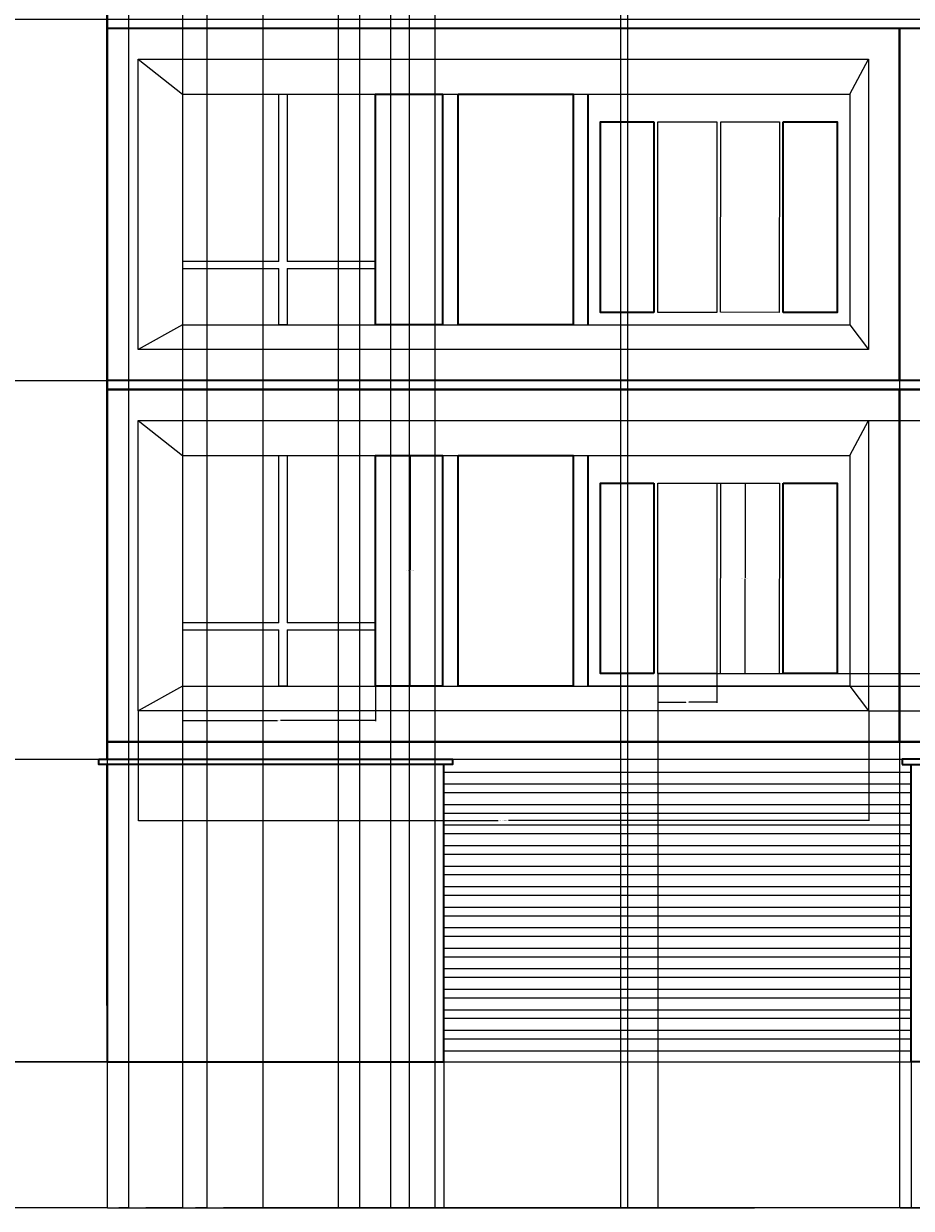
# Model space of a CAD drawing. Units: feet. Extents: x 1141 to 2858, y 751 to 1654.
# Tile 9 of 13: x 2288 to 2621, y 751 to 1195. Entities that reach past the tile are written whole.
import ezdxf

# ---------------------------------------------------------------- set-up
doc = ezdxf.new("R2010")
doc.units = ezdxf.units.FT
for name, color, linetype, lineweight in [('A-ANNO-DIMS', 2, 'Continuous', 18), ('A-DOOR', 3, 'Continuous', 25), ('A-ELEV', 7, 'Continuous', 35), ('A-GLAZ', 4, 'Continuous', 25)]:
    doc.layers.add(name, color=color, linetype=linetype, lineweight=lineweight)
doc.styles.get("Standard").update_dxf_attribs({"font": 'arial.ttf'})
doc.dimstyles.get("Standard").update_dxf_attribs({"dimtxt": 0.18, "dimasz": 0.18, "dimexe": 0.18, "dimexo": 0.0625, "dimgap": 0.09, "dimtad": 0, "dimtih": 1, "dimtoh": 1, "dimdec": 1, "dimzin": 0, "dimdsep": 46, "dimlunit": 3, "dimtxsty": 'Standard', "dimcen": 0.09, "dimadec": 0, "dimazin": 0, "dimtfac": 1, "dimtdec": 1, "dimtofl": 0, "dimtmove": 0, "dimatfit": 3, "dimfxl": 1, "dimtolj": 1, "dimtzin": 0, "dimarcsym": 0})

# ---------------------------------------------------------------- blocks, each defined once
blk = doc.blocks.new('BALCONY-GLAZ-B')
for p, q in [((0, 108.84), (16.63, 95.74)), ((266.62, 95.74), (273.67, 108.84)), ((16.63, 95.74), (16.63, 9.29)), ((16.63, 95.74), (266.62, 95.74)), ((266.62, 95.74), (266.62, 9.19)), ((16.63, 9.29), (0, 0)), ((16.63, 9.29), (266.62, 9.29)), ((266.62, 9.29), (273.67, 0))]:
    blk.add_line(p, q)
for points in [[(0, 108.84), (273.67, 108.84), (273.67, 0), (0, 0)], [(266.62, 9.19), (168.47, 9.19), (168.47, 95.74), (266.62, 95.74)]]:
    blk.add_lwpolyline(points, close=True)
blk = doc.blocks.new('WIN-SLIDING')
for points in [[(36.16, 23.71), (36.16, 86.44), (39.2, 86.44), (39.2, 23.71)], [(36.16, 23.71), (0, 23.71), (0, 21.05), (36.16, 21.05)], [(39.2, 21.05), (72.32, 21.05), (72.32, 23.71), (39.2, 23.71)], [(39.2, 21.05), (39.2, 0), (36.16, 0), (36.16, 21.05)]]:
    blk.add_lwpolyline(points)
blk = doc.blocks.new('GLAZ-PANEL-B')
for points in [[(0, 71.37), (22, 71.37)], [(0, 0), (0, 71.37)], [(22, 71.37), (22, 0)], [(22, 0), (0, 0)]]:
    blk.add_lwpolyline(points)
blk = doc.blocks.new('*D8')
at = {"layer": 'A-ANNO-DIMS', "color": 0, "lineweight": -2, "transparency": 16777216}
for p, q in [((2419.9, 1033.22), (2432.98, 1033.22)), ((2432.8, 1033.04), (2432.8, 990.18)), ((2432.8, 946.95), (2432.8, 989.81)), ((2419.9, 946.77), (2432.98, 946.77))]:
    blk.add_line(p, q, dxfattribs=at)
at = {"layer": 'A-ANNO-DIMS', "color": 0, "transparency": 16777216}
for points in [[(2432.77, 1033.04), (2432.83, 1033.04), (2432.8, 1033.22)], [(2432.77, 946.95), (2432.83, 946.95), (2432.8, 946.77)]]:
    blk.add_solid(points, dxfattribs=at)
at = {"layer": 'Defpoints', "color": 0, "transparency": 16777216}
for p in [(2419.84, 1033.22), (2432.8, 1033.22), (2419.84, 946.77)]:
    blk.add_point(p, dxfattribs=at)
at = {"layer": 'A-ANNO-DIMS', "color": 0, "transparency": 16777216, "insert": (2432.8, 990), "char_height": 0.18, "attachment_point": 5}
blk.add_mtext('\\A1;SLIDING WINDOW 86 TYP.', dxfattribs=at)
blk = doc.blocks.new('*D9')
at = {"layer": 'A-ANNO-DIMS', "color": 0, "lineweight": -2, "transparency": 16777216}
for p, q in [((2347.51, 946.71), (2347.51, 933.63)), ((2419.84, 946.71), (2419.84, 933.63)), ((2347.69, 933.81), (2383.15, 933.81)), ((2419.66, 933.81), (2384.2, 933.81))]:
    blk.add_line(p, q, dxfattribs=at)
at = {"layer": 'A-ANNO-DIMS', "color": 0, "transparency": 16777216}
for points in [[(2347.69, 933.84), (2347.69, 933.78), (2347.51, 933.81)], [(2419.66, 933.84), (2419.66, 933.78), (2419.84, 933.81)]]:
    blk.add_solid(points, dxfattribs=at)
at = {"layer": 'Defpoints', "color": 0, "transparency": 16777216}
for p in [(2347.51, 946.77), (2419.84, 946.77), (2419.84, 933.81)]:
    blk.add_point(p, dxfattribs=at)
at = {"layer": 'A-ANNO-DIMS', "color": 0, "transparency": 16777216, "insert": (2383.67, 933.81), "char_height": 0.18, "attachment_point": 5}
blk.add_mtext('\\A1;72 TYP.', dxfattribs=at)
blk = doc.blocks.new('*D12')
at = {"layer": 'A-ANNO-DIMS', "color": 0, "lineweight": -2, "transparency": 16777216}
for p, q in [((2547.7, 1022.8), (2558.53, 1022.8)), ((2558.35, 1022.62), (2558.35, 987.3)), ((2558.35, 951.61), (2558.35, 986.93)), ((2547.7, 951.43), (2558.53, 951.43))]:
    blk.add_line(p, q, dxfattribs=at)
at = {"layer": 'A-ANNO-DIMS', "color": 0, "transparency": 16777216}
for points in [[(2558.32, 1022.62), (2558.38, 1022.62), (2558.35, 1022.8)], [(2558.32, 951.61), (2558.38, 951.61), (2558.35, 951.43)]]:
    blk.add_solid(points, dxfattribs=at)
at = {"layer": 'Defpoints', "color": 0, "transparency": 16777216}
for p in [(2547.64, 1022.8), (2558.35, 1022.8), (2547.64, 951.43)]:
    blk.add_point(p, dxfattribs=at)
at = {"layer": 'A-ANNO-DIMS', "color": 0, "transparency": 16777216, "insert": (2558.35, 987.11), "char_height": 0.18, "attachment_point": 5}
blk.add_mtext('\\A1;GLAZING PANEL B 71 TYP.', dxfattribs=at)
blk = doc.blocks.new('*D13')
at = {"layer": 'A-ANNO-DIMS', "color": 0, "lineweight": -2, "transparency": 16777216}
for p, q in [((2525.64, 951.37), (2525.64, 940.54)), ((2547.64, 951.37), (2547.64, 940.54)), ((2525.82, 940.72), (2536.11, 940.72)), ((2547.46, 940.72), (2537.17, 940.72))]:
    blk.add_line(p, q, dxfattribs=at)
at = {"layer": 'A-ANNO-DIMS', "color": 0, "transparency": 16777216}
for points in [[(2525.82, 940.75), (2525.82, 940.69), (2525.64, 940.72)], [(2547.46, 940.75), (2547.46, 940.69), (2547.64, 940.72)]]:
    blk.add_solid(points, dxfattribs=at)
at = {"layer": 'Defpoints', "color": 0, "transparency": 16777216}
for p in [(2525.64, 951.43), (2547.64, 951.43), (2547.64, 940.72)]:
    blk.add_point(p, dxfattribs=at)
at = {"layer": 'A-ANNO-DIMS', "color": 0, "transparency": 16777216, "insert": (2536.64, 940.72), "char_height": 0.18, "attachment_point": 5}
blk.add_mtext('\\A1;22 TYP.', dxfattribs=at)
blk = doc.blocks.new('*D20')
at = {"layer": 'A-ANNO-DIMS', "color": 0, "lineweight": -2, "transparency": 16777216}
for p, q in [((2330.88, 937.42), (2330.88, 896.25)), ((2604.56, 937.42), (2604.56, 896.25)), ((2331.06, 896.43), (2465.78, 896.43)), ((2604.38, 896.43), (2469.65, 896.43))]:
    blk.add_line(p, q, dxfattribs=at)
at = {"layer": 'A-ANNO-DIMS', "color": 0, "transparency": 16777216}
for points in [[(2331.06, 896.46), (2331.06, 896.4), (2330.88, 896.43)], [(2604.38, 896.46), (2604.38, 896.4), (2604.56, 896.43)]]:
    blk.add_solid(points, dxfattribs=at)
at = {"layer": 'Defpoints', "color": 0, "transparency": 16777216}
for p in [(2330.88, 937.48), (2604.56, 937.48), (2604.56, 896.43)]:
    blk.add_point(p, dxfattribs=at)
at = {"layer": 'A-ANNO-DIMS', "color": 0, "transparency": 16777216, "insert": (2467.72, 896.43), "char_height": 0.18, "attachment_point": 5}
blk.add_mtext('\\A1;BALCONY GLAZING B 274 TYP.', dxfattribs=at)
blk = doc.blocks.new('*D21')
at = {"layer": 'A-ANNO-DIMS', "color": 0, "lineweight": -2, "transparency": 16777216}
for p, q in [((2604.62, 1046.32), (2645.79, 1046.32)), ((2645.61, 1046.14), (2645.61, 992.08)), ((2645.61, 937.66), (2645.61, 991.72)), ((2604.62, 937.48), (2645.79, 937.48))]:
    blk.add_line(p, q, dxfattribs=at)
at = {"layer": 'A-ANNO-DIMS', "color": 0, "transparency": 16777216}
for points in [[(2645.58, 1046.14), (2645.64, 1046.14), (2645.61, 1046.32)], [(2645.58, 937.66), (2645.64, 937.66), (2645.61, 937.48)]]:
    blk.add_solid(points, dxfattribs=at)
at = {"layer": 'Defpoints', "color": 0, "transparency": 16777216}
for p in [(2604.56, 1046.32), (2645.61, 1046.32), (2604.56, 937.48)]:
    blk.add_point(p, dxfattribs=at)
at = {"layer": 'A-ANNO-DIMS', "color": 0, "transparency": 16777216, "insert": (2645.61, 991.9), "char_height": 0.18, "attachment_point": 5}
blk.add_mtext('\\A1;109 TYP.', dxfattribs=at)
blk = doc.blocks.new('*D23')
at = {"layer": 'A-ANNO-DIMS', "color": 0, "lineweight": -2, "transparency": 16777216}
for p, q in [((2206.03, 805.84), (2206.03, 751.07)), ((2319.3, 805.84), (2319.3, 751.07)), ((2206.21, 751.25), (2262.21, 751.25)), ((2319.12, 751.25), (2263.12, 751.25))]:
    blk.add_line(p, q, dxfattribs=at)
at = {"layer": 'A-ANNO-DIMS', "color": 0, "transparency": 16777216}
for points in [[(2206.21, 751.28), (2206.21, 751.22), (2206.03, 751.25)], [(2319.12, 751.28), (2319.12, 751.22), (2319.3, 751.25)]]:
    blk.add_solid(points, dxfattribs=at)
at = {"layer": 'Defpoints', "color": 0, "transparency": 16777216}
for p in [(2206.03, 805.9), (2319.3, 805.9), (2319.3, 751.25)]:
    blk.add_point(p, dxfattribs=at)
at = {"layer": 'A-ANNO-DIMS', "color": 0, "transparency": 16777216, "insert": (2262.67, 751.25), "char_height": 0.18, "attachment_point": 5}
blk.add_mtext('\\A1;113.27', dxfattribs=at)
blk = doc.blocks.new('*D29')
at = {"layer": 'A-ANNO-DIMS', "color": 0, "lineweight": -2, "transparency": 16777216}
for p, q in [((2206.09, 919.34), (2857.83, 919.34)), ((2857.65, 919.16), (2857.65, 862.8)), ((2857.65, 806.08), (2857.65, 862.44)), ((2206.09, 805.9), (2857.83, 805.9))]:
    blk.add_line(p, q, dxfattribs=at)
at = {"layer": 'A-ANNO-DIMS', "color": 0, "transparency": 16777216}
for points in [[(2857.62, 919.16), (2857.68, 919.16), (2857.65, 919.34)], [(2857.62, 806.08), (2857.68, 806.08), (2857.65, 805.9)]]:
    blk.add_solid(points, dxfattribs=at)
at = {"layer": 'Defpoints', "color": 0, "transparency": 16777216}
for p in [(2206.03, 919.34), (2857.65, 919.34), (2206.03, 805.9)]:
    blk.add_point(p, dxfattribs=at)
at = {"layer": 'A-ANNO-DIMS', "color": 0, "transparency": 16777216, "insert": (2857.65, 862.62), "char_height": 0.18, "attachment_point": 5}
blk.add_mtext('\\A1;113.44', dxfattribs=at)
blk = doc.blocks.new('*D30')
at = {"layer": 'A-ANNO-DIMS', "color": 0, "lineweight": -2, "transparency": 16777216}
for p, q in [((2117.47, 1061.29), (2857.83, 1061.29)), ((2857.65, 1061.11), (2857.65, 990.5)), ((2857.65, 919.52), (2857.65, 990.13)), ((2117.47, 919.34), (2857.83, 919.34))]:
    blk.add_line(p, q, dxfattribs=at)
at = {"layer": 'A-ANNO-DIMS', "color": 0, "transparency": 16777216}
for points in [[(2857.62, 1061.11), (2857.68, 1061.11), (2857.65, 1061.29)], [(2857.62, 919.52), (2857.68, 919.52), (2857.65, 919.34)]]:
    blk.add_solid(points, dxfattribs=at)
at = {"layer": 'Defpoints', "color": 0, "transparency": 16777216}
for p in [(2117.41, 1061.29), (2857.65, 1061.29), (2117.41, 919.34)]:
    blk.add_point(p, dxfattribs=at)
at = {"layer": 'A-ANNO-DIMS', "color": 0, "transparency": 16777216, "insert": (2857.65, 990.31), "char_height": 0.18, "attachment_point": 5}
blk.add_mtext('\\A1;141.95', dxfattribs=at)
blk = doc.blocks.new('*D31')
at = {"layer": 'A-ANNO-DIMS', "color": 0, "lineweight": -2, "transparency": 16777216}
for p, q in [((2117.47, 1196.68), (2857.83, 1196.68)), ((2857.65, 1196.5), (2857.65, 1129.16)), ((2857.65, 1061.47), (2857.65, 1128.8)), ((2117.47, 1061.29), (2857.83, 1061.29))]:
    blk.add_line(p, q, dxfattribs=at)
at = {"layer": 'A-ANNO-DIMS', "color": 0, "transparency": 16777216}
for points in [[(2857.62, 1196.5), (2857.68, 1196.5), (2857.65, 1196.68)], [(2857.62, 1061.47), (2857.68, 1061.47), (2857.65, 1061.29)]]:
    blk.add_solid(points, dxfattribs=at)
at = {"layer": 'Defpoints', "color": 0, "transparency": 16777216}
for p in [(2117.41, 1196.68), (2857.65, 1196.68), (2117.41, 1061.29)]:
    blk.add_point(p, dxfattribs=at)
at = {"layer": 'A-ANNO-DIMS', "color": 0, "transparency": 16777216, "insert": (2857.65, 1128.98), "char_height": 0.18, "attachment_point": 5}
blk.add_mtext('\\A1;135.4', dxfattribs=at)
blk = doc.blocks.new('*D36')
at = {"layer": 'A-ANNO-DIMS', "color": 0, "lineweight": -2, "transparency": 16777216}
for p, q in [((2319.3, 805.84), (2319.3, 751.07)), ((2445.45, 805.84), (2445.45, 751.07)), ((2319.48, 751.25), (2381.92, 751.25)), ((2445.27, 751.25), (2382.83, 751.25))]:
    blk.add_line(p, q, dxfattribs=at)
at = {"layer": 'A-ANNO-DIMS', "color": 0, "transparency": 16777216}
for points in [[(2319.48, 751.28), (2319.48, 751.22), (2319.3, 751.25)], [(2445.27, 751.28), (2445.27, 751.22), (2445.45, 751.25)]]:
    blk.add_solid(points, dxfattribs=at)
at = {"layer": 'Defpoints', "color": 0, "transparency": 16777216}
for p in [(2319.3, 805.9), (2445.45, 805.9), (2445.45, 751.25)]:
    blk.add_point(p, dxfattribs=at)
at = {"layer": 'A-ANNO-DIMS', "color": 0, "transparency": 16777216, "insert": (2382.37, 751.25), "char_height": 0.18, "attachment_point": 5}
blk.add_mtext('\\A1;126.15', dxfattribs=at)
blk = doc.blocks.new('*D37')
at = {"layer": 'A-ANNO-DIMS', "color": 0, "lineweight": -2, "transparency": 16777216}
for p, q in [((2445.45, 805.84), (2445.45, 751.07)), ((2620.53, 805.84), (2620.53, 751.07)), ((2445.63, 751.25), (2532.53, 751.25)), ((2620.35, 751.25), (2533.44, 751.25))]:
    blk.add_line(p, q, dxfattribs=at)
at = {"layer": 'A-ANNO-DIMS', "color": 0, "transparency": 16777216}
for points in [[(2445.63, 751.28), (2445.63, 751.22), (2445.45, 751.25)], [(2620.35, 751.28), (2620.35, 751.22), (2620.53, 751.25)]]:
    blk.add_solid(points, dxfattribs=at)
at = {"layer": 'Defpoints', "color": 0, "transparency": 16777216}
for p in [(2445.45, 805.9), (2620.53, 805.9), (2620.53, 751.25)]:
    blk.add_point(p, dxfattribs=at)
at = {"layer": 'A-ANNO-DIMS', "color": 0, "transparency": 16777216, "insert": (2532.99, 751.25), "char_height": 0.18, "attachment_point": 5}
blk.add_mtext('\\A1;175.08', dxfattribs=at)
blk = doc.blocks.new('*D39')
at = {"layer": 'A-ANNO-DIMS', "color": 0, "lineweight": -2, "transparency": 16777216}
for p, q in [((2319.24, 1599.45), (1668.14, 1599.45)), ((1668.32, 1599.27), (1668.32, 1202.86)), ((1668.32, 806.08), (1668.32, 1202.49)), ((2319.24, 805.9), (1668.14, 805.9))]:
    blk.add_line(p, q, dxfattribs=at)
at = {"layer": 'A-ANNO-DIMS', "color": 0, "transparency": 16777216}
for points in [[(1668.29, 1599.27), (1668.35, 1599.27), (1668.32, 1599.45)], [(1668.29, 806.08), (1668.35, 806.08), (1668.32, 805.9)]]:
    blk.add_solid(points, dxfattribs=at)
at = {"layer": 'Defpoints', "color": 0, "transparency": 16777216}
for p in [(1668.32, 1599.45), (2319.3, 1599.45), (2319.3, 805.9)]:
    blk.add_point(p, dxfattribs=at)
at = {"layer": 'A-ANNO-DIMS', "color": 0, "transparency": 16777216, "insert": (1668.32, 1202.68), "char_height": 0.18, "attachment_point": 5}
blk.add_mtext('\\A1;793.6', dxfattribs=at)
blk = doc.blocks.new('*D40')
at = {"layer": 'A-ANNO-DIMS', "color": 0, "lineweight": -2, "transparency": 16777216}
for p, q in [((2319.3, 1193.23), (2319.3, 751.07)), ((2616.14, 1193.23), (2616.14, 751.07)), ((2319.48, 751.25), (2467.25, 751.25)), ((2615.96, 751.25), (2468.18, 751.25))]:
    blk.add_line(p, q, dxfattribs=at)
at = {"layer": 'A-ANNO-DIMS', "color": 0, "transparency": 16777216}
for points in [[(2319.48, 751.28), (2319.48, 751.22), (2319.3, 751.25)], [(2615.96, 751.28), (2615.96, 751.22), (2616.14, 751.25)]]:
    blk.add_solid(points, dxfattribs=at)
at = {"layer": 'Defpoints', "color": 0, "transparency": 16777216}
for p in [(2319.3, 1193.29), (2616.14, 1193.29), (2616.14, 751.25)]:
    blk.add_point(p, dxfattribs=at)
at = {"layer": 'A-ANNO-DIMS', "color": 0, "transparency": 16777216, "insert": (2467.72, 751.25), "char_height": 0.18, "attachment_point": 5}
blk.add_mtext('\\A1;296.83', dxfattribs=at)
blk = doc.blocks.new('*D41')
at = {"layer": 'A-ANNO-DIMS', "color": 0, "lineweight": -2, "transparency": 16777216}
for p, q in [((2616.14, 1193.23), (2616.14, 751.07)), ((2710.68, 1193.23), (2710.68, 751.07)), ((2616.32, 751.25), (2663.01, 751.25)), ((2710.5, 751.25), (2663.8, 751.25))]:
    blk.add_line(p, q, dxfattribs=at)
at = {"layer": 'A-ANNO-DIMS', "color": 0, "transparency": 16777216}
for points in [[(2616.32, 751.28), (2616.32, 751.22), (2616.14, 751.25)], [(2710.5, 751.28), (2710.5, 751.22), (2710.68, 751.25)]]:
    blk.add_solid(points, dxfattribs=at)
at = {"layer": 'Defpoints', "color": 0, "transparency": 16777216}
for p in [(2616.14, 1193.29), (2710.68, 1193.29), (2710.68, 751.25)]:
    blk.add_point(p, dxfattribs=at)
at = {"layer": 'A-ANNO-DIMS', "color": 0, "transparency": 16777216, "insert": (2663.41, 751.25), "char_height": 0.18, "attachment_point": 5}
blk.add_mtext('\\A1;94.54', dxfattribs=at)
blk = doc.blocks.new('*D55')
at = {"layer": 'A-ANNO-DIMS', "color": 0, "lineweight": -2, "transparency": 16777216}
for p, q in [((2347.51, 1574.71), (2347.51, 751.07)), ((2356.64, 1548.48), (2356.64, 751.07)), ((2347.69, 751.25), (2351.75, 751.25)), ((2356.46, 751.25), (2352.4, 751.25))]:
    blk.add_line(p, q, dxfattribs=at)
at = {"layer": 'A-ANNO-DIMS', "color": 0, "transparency": 16777216}
for points in [[(2347.69, 751.28), (2347.69, 751.22), (2347.51, 751.25)], [(2356.46, 751.28), (2356.46, 751.22), (2356.64, 751.25)]]:
    blk.add_solid(points, dxfattribs=at)
at = {"layer": 'Defpoints', "color": 0, "transparency": 16777216}
for p in [(2347.51, 1574.77), (2356.64, 1548.54), (2356.64, 751.25)]:
    blk.add_point(p, dxfattribs=at)
at = {"layer": 'A-ANNO-DIMS', "color": 0, "transparency": 16777216, "insert": (2352.08, 751.25), "char_height": 0.18, "attachment_point": 5}
blk.add_mtext('\\A1;9.13', dxfattribs=at)
blk = doc.blocks.new('*D61')
at = {"layer": 'A-ANNO-DIMS', "color": 0, "lineweight": -2, "transparency": 16777216}
for p, q in [((2347.51, 1488.26), (2347.51, 751.07)), ((2377.6, 1488.26), (2377.6, 751.07)), ((2347.69, 751.25), (2362.16, 751.25)), ((2377.42, 751.25), (2362.95, 751.25))]:
    blk.add_line(p, q, dxfattribs=at)
at = {"layer": 'A-ANNO-DIMS', "color": 0, "transparency": 16777216}
for points in [[(2347.69, 751.28), (2347.69, 751.22), (2347.51, 751.25)], [(2377.42, 751.28), (2377.42, 751.22), (2377.6, 751.25)]]:
    blk.add_solid(points, dxfattribs=at)
at = {"layer": 'Defpoints', "color": 0, "transparency": 16777216}
for p in [(2347.51, 1488.33), (2377.6, 1488.33), (2377.6, 751.25)]:
    blk.add_point(p, dxfattribs=at)
at = {"layer": 'A-ANNO-DIMS', "color": 0, "transparency": 16777216, "insert": (2362.56, 751.25), "char_height": 0.18, "attachment_point": 5}
blk.add_mtext('\\A1;30.09', dxfattribs=at)
blk = doc.blocks.new('*D62')
at = {"layer": 'A-ANNO-DIMS', "color": 0, "lineweight": -2, "transparency": 16777216}
for p, q in [((2377.6, 1488.26), (2377.6, 751.07)), ((2442.01, 1488.26), (2442.01, 751.07)), ((2377.78, 751.25), (2409.48, 751.25)), ((2441.83, 751.25), (2410.13, 751.25))]:
    blk.add_line(p, q, dxfattribs=at)
at = {"layer": 'A-ANNO-DIMS', "color": 0, "transparency": 16777216}
for points in [[(2377.78, 751.28), (2377.78, 751.22), (2377.6, 751.25)], [(2441.83, 751.28), (2441.83, 751.22), (2442.01, 751.25)]]:
    blk.add_solid(points, dxfattribs=at)
at = {"layer": 'Defpoints', "color": 0, "transparency": 16777216}
for p in [(2377.6, 1488.33), (2442.01, 1488.33), (2442.01, 751.25)]:
    blk.add_point(p, dxfattribs=at)
at = {"layer": 'A-ANNO-DIMS', "color": 0, "transparency": 16777216, "insert": (2409.81, 751.25), "char_height": 0.18, "attachment_point": 5}
blk.add_mtext('\\A1;64.4', dxfattribs=at)
blk = doc.blocks.new('*D63')
at = {"layer": 'A-ANNO-DIMS', "color": 0, "lineweight": -2, "transparency": 16777216}
for p, q in [((2511.62, 1488.26), (2511.62, 751.07)), ((2514.19, 1488.26), (2514.19, 751.07)), ((2511.8, 751.25), (2512.58, 751.25)), ((2514.01, 751.25), (2513.23, 751.25))]:
    blk.add_line(p, q, dxfattribs=at)
at = {"layer": 'A-ANNO-DIMS', "color": 0, "transparency": 16777216}
for points in [[(2511.8, 751.28), (2511.8, 751.22), (2511.62, 751.25)], [(2514.01, 751.28), (2514.01, 751.22), (2514.19, 751.25)]]:
    blk.add_solid(points, dxfattribs=at)
at = {"layer": 'Defpoints', "color": 0, "transparency": 16777216}
for p in [(2511.62, 1488.33), (2514.19, 1488.33), (2514.19, 751.25)]:
    blk.add_point(p, dxfattribs=at)
at = {"layer": 'A-ANNO-DIMS', "color": 0, "transparency": 16777216, "insert": (2512.91, 751.25), "char_height": 0.18, "attachment_point": 5}
blk.add_mtext('\\A1;2.57', dxfattribs=at)
blk = doc.blocks.new('*D67')
at = {"layer": 'A-ANNO-DIMS', "color": 0, "lineweight": -2, "transparency": 16777216}
for p, q in [((2327.29, 1339.99), (2327.29, 751.07)), ((2319.3, 1332), (2319.3, 751.07)), ((2319.48, 751.25), (2322.9, 751.25)), ((2327.11, 751.25), (2323.69, 751.25))]:
    blk.add_line(p, q, dxfattribs=at)
at = {"layer": 'A-ANNO-DIMS', "color": 0, "transparency": 16777216}
for points in [[(2319.48, 751.28), (2319.48, 751.22), (2319.3, 751.25)], [(2327.11, 751.28), (2327.11, 751.22), (2327.29, 751.25)]]:
    blk.add_solid(points, dxfattribs=at)
at = {"layer": 'Defpoints', "color": 0, "transparency": 16777216}
for p in [(2327.29, 1340.05), (2319.3, 1332.06), (2327.29, 751.25)]:
    blk.add_point(p, dxfattribs=at)
at = {"layer": 'A-ANNO-DIMS', "color": 0, "transparency": 16777216, "insert": (2323.29, 751.25), "char_height": 0.18, "attachment_point": 5}
blk.add_mtext('\\A1;7.986', dxfattribs=at)
blk = doc.blocks.new('*D68')
at = {"layer": 'A-ANNO-DIMS', "color": 0, "lineweight": -2, "transparency": 16777216}
for p, q in [((2405.86, 1339.99), (2405.86, 751.07)), ((2413.84, 1332), (2413.84, 751.07)), ((2406.04, 751.25), (2409.46, 751.25)), ((2413.66, 751.25), (2410.24, 751.25))]:
    blk.add_line(p, q, dxfattribs=at)
at = {"layer": 'A-ANNO-DIMS', "color": 0, "transparency": 16777216}
for points in [[(2406.04, 751.28), (2406.04, 751.22), (2405.86, 751.25)], [(2413.66, 751.28), (2413.66, 751.22), (2413.84, 751.25)]]:
    blk.add_solid(points, dxfattribs=at)
at = {"layer": 'Defpoints', "color": 0, "transparency": 16777216}
for p in [(2405.86, 1340.05), (2413.84, 1332.06), (2413.84, 751.25)]:
    blk.add_point(p, dxfattribs=at)
at = {"layer": 'A-ANNO-DIMS', "color": 0, "transparency": 16777216, "insert": (2409.85, 751.25), "char_height": 0.18, "attachment_point": 5}
blk.add_mtext('\\A1;7.986', dxfattribs=at)
blk = doc.blocks.new('*D69')
at = {"layer": 'A-ANNO-DIMS', "color": 0, "lineweight": -2, "transparency": 16777216}
for p, q in [((2425.42, 1343.58), (2425.42, 751.07)), ((2413.84, 1332), (2413.84, 751.07)), ((2414.02, 751.25), (2419.25, 751.25)), ((2425.24, 751.25), (2420.02, 751.25))]:
    blk.add_line(p, q, dxfattribs=at)
at = {"layer": 'A-ANNO-DIMS', "color": 0, "transparency": 16777216}
for points in [[(2414.02, 751.28), (2414.02, 751.22), (2413.84, 751.25)], [(2425.24, 751.28), (2425.24, 751.22), (2425.42, 751.25)]]:
    blk.add_solid(points, dxfattribs=at)
at = {"layer": 'Defpoints', "color": 0, "transparency": 16777216}
for p in [(2425.42, 1343.65), (2413.84, 1332.06), (2425.42, 751.25)]:
    blk.add_point(p, dxfattribs=at)
at = {"layer": 'A-ANNO-DIMS', "color": 0, "transparency": 16777216, "insert": (2419.63, 751.25), "char_height": 0.18, "attachment_point": 5}
blk.add_mtext('\\A1;11.58', dxfattribs=at)
blk = doc.blocks.new('*D70')
at = {"layer": 'A-ANNO-DIMS', "color": 0, "lineweight": -2, "transparency": 16777216}
for p, q in [((2432.48, 1352.88), (2432.48, 751.07)), ((2425.42, 1343.58), (2425.42, 751.07)), ((2425.6, 751.25), (2428.56, 751.25)), ((2432.3, 751.25), (2429.34, 751.25))]:
    blk.add_line(p, q, dxfattribs=at)
at = {"layer": 'A-ANNO-DIMS', "color": 0, "transparency": 16777216}
for points in [[(2425.6, 751.28), (2425.6, 751.22), (2425.42, 751.25)], [(2432.3, 751.28), (2432.3, 751.22), (2432.48, 751.25)]]:
    blk.add_solid(points, dxfattribs=at)
at = {"layer": 'Defpoints', "color": 0, "transparency": 16777216}
for p in [(2432.48, 1352.94), (2425.42, 1343.65), (2432.48, 751.25)]:
    blk.add_point(p, dxfattribs=at)
at = {"layer": 'A-ANNO-DIMS', "color": 0, "transparency": 16777216, "insert": (2428.95, 751.25), "char_height": 0.18, "attachment_point": 5}
blk.add_mtext('\\A1;7.054', dxfattribs=at)
blk = doc.blocks.new('*D73')
at = {"layer": 'A-ANNO-DIMS', "color": 0, "lineweight": -2, "transparency": 16777216}
for p, q in [((2319.3, 1332), (2319.3, 751.07)), ((2413.84, 1332), (2413.84, 751.07)), ((2319.48, 751.25), (2366.18, 751.25)), ((2413.66, 751.25), (2366.96, 751.25))]:
    blk.add_line(p, q, dxfattribs=at)
at = {"layer": 'A-ANNO-DIMS', "color": 0, "transparency": 16777216}
for points in [[(2319.48, 751.28), (2319.48, 751.22), (2319.3, 751.25)], [(2413.66, 751.28), (2413.66, 751.22), (2413.84, 751.25)]]:
    blk.add_solid(points, dxfattribs=at)
at = {"layer": 'Defpoints', "color": 0, "transparency": 16777216}
for p in [(2319.3, 1332.06), (2413.84, 1332.06), (2413.84, 751.25)]:
    blk.add_point(p, dxfattribs=at)
at = {"layer": 'A-ANNO-DIMS', "color": 0, "transparency": 16777216, "insert": (2366.57, 751.25), "char_height": 0.18, "attachment_point": 5}
blk.add_mtext('\\A1;94.54', dxfattribs=at)
blk = doc.blocks.new('*D74')
at = {"layer": 'A-ANNO-DIMS', "color": 0, "lineweight": -2, "transparency": 16777216}
for p, q in [((2413.84, 1332), (2413.84, 751.07)), ((2710.68, 1332), (2710.68, 751.07)), ((2414.02, 751.25), (2561.79, 751.25)), ((2710.5, 751.25), (2562.72, 751.25))]:
    blk.add_line(p, q, dxfattribs=at)
at = {"layer": 'A-ANNO-DIMS', "color": 0, "transparency": 16777216}
for points in [[(2414.02, 751.28), (2414.02, 751.22), (2413.84, 751.25)], [(2710.5, 751.28), (2710.5, 751.22), (2710.68, 751.25)]]:
    blk.add_solid(points, dxfattribs=at)
at = {"layer": 'Defpoints', "color": 0, "transparency": 16777216}
for p in [(2413.84, 1332.06), (2710.68, 1332.06), (2710.68, 751.25)]:
    blk.add_point(p, dxfattribs=at)
at = {"layer": 'A-ANNO-DIMS', "color": 0, "transparency": 16777216, "insert": (2562.26, 751.25), "char_height": 0.18, "attachment_point": 5}
blk.add_mtext('\\A1;296.83', dxfattribs=at)
blk = doc.blocks.new('*D78')
at = {"layer": 'A-ANNO-DIMS', "color": 0, "lineweight": -2, "transparency": 16777216}
for p, q in [((2347.51, 946.71), (2347.51, 751.07)), ((2319.3, 919.28), (2319.3, 751.07)), ((2319.48, 751.25), (2333.03, 751.25)), ((2347.33, 751.25), (2333.78, 751.25))]:
    blk.add_line(p, q, dxfattribs=at)
at = {"layer": 'A-ANNO-DIMS', "color": 0, "transparency": 16777216}
for points in [[(2319.48, 751.28), (2319.48, 751.22), (2319.3, 751.25)], [(2347.33, 751.28), (2347.33, 751.22), (2347.51, 751.25)]]:
    blk.add_solid(points, dxfattribs=at)
at = {"layer": 'Defpoints', "color": 0, "transparency": 16777216}
for p in [(2347.51, 946.77), (2319.3, 919.34), (2347.51, 751.25)]:
    blk.add_point(p, dxfattribs=at)
at = {"layer": 'A-ANNO-DIMS', "color": 0, "transparency": 16777216, "insert": (2333.41, 751.25), "char_height": 0.18, "attachment_point": 5}
blk.add_mtext('\\A1;28.21', dxfattribs=at)
blk = doc.blocks.new('*D79')
at = {"layer": 'A-ANNO-DIMS', "color": 0, "lineweight": -2, "transparency": 16777216}
for p, q in [((2525.64, 951.37), (2525.64, 751.07)), ((2319.3, 919.28), (2319.3, 751.07)), ((2319.48, 751.25), (2422.01, 751.25)), ((2525.46, 751.25), (2422.94, 751.25))]:
    blk.add_line(p, q, dxfattribs=at)
at = {"layer": 'A-ANNO-DIMS', "color": 0, "transparency": 16777216}
for points in [[(2319.48, 751.28), (2319.48, 751.22), (2319.3, 751.25)], [(2525.46, 751.28), (2525.46, 751.22), (2525.64, 751.25)]]:
    blk.add_solid(points, dxfattribs=at)
at = {"layer": 'Defpoints', "color": 0, "transparency": 16777216}
for p in [(2525.64, 951.43), (2319.3, 919.34), (2525.64, 751.25)]:
    blk.add_point(p, dxfattribs=at)
at = {"layer": 'A-ANNO-DIMS', "color": 0, "transparency": 16777216, "insert": (2422.47, 751.25), "char_height": 0.18, "attachment_point": 5}
blk.add_mtext('\\A1;206.34', dxfattribs=at)
blk = doc.blocks.new('*D80')
at = {"layer": 'A-ANNO-DIMS', "color": 0, "lineweight": -2, "transparency": 16777216}
for p, q in [((2347.57, 946.77), (2857.83, 946.77)), ((2857.65, 946.59), (2857.65, 933.24)), ((2857.65, 919.52), (2857.65, 932.87)), ((2319.36, 919.34), (2857.83, 919.34))]:
    blk.add_line(p, q, dxfattribs=at)
at = {"layer": 'A-ANNO-DIMS', "color": 0, "transparency": 16777216}
for points in [[(2857.62, 946.59), (2857.68, 946.59), (2857.65, 946.77)], [(2857.62, 919.52), (2857.68, 919.52), (2857.65, 919.34)]]:
    blk.add_solid(points, dxfattribs=at)
at = {"layer": 'Defpoints', "color": 0, "transparency": 16777216}
for p in [(2347.51, 946.77), (2857.65, 946.77), (2319.3, 919.34)]:
    blk.add_point(p, dxfattribs=at)
at = {"layer": 'A-ANNO-DIMS', "color": 0, "transparency": 16777216, "insert": (2857.65, 933.06), "char_height": 0.18, "attachment_point": 5}
blk.add_mtext('\\A1;27.435', dxfattribs=at)
blk = doc.blocks.new('*D81')
at = {"layer": 'A-ANNO-DIMS', "color": 0, "lineweight": -2, "transparency": 16777216}
for p, q in [((2525.7, 951.43), (2857.83, 951.43)), ((2857.65, 951.25), (2857.65, 935.57)), ((2857.65, 919.52), (2857.65, 935.2)), ((2319.36, 919.34), (2857.83, 919.34))]:
    blk.add_line(p, q, dxfattribs=at)
at = {"layer": 'A-ANNO-DIMS', "color": 0, "transparency": 16777216}
for points in [[(2857.62, 951.25), (2857.68, 951.25), (2857.65, 951.43)], [(2857.62, 919.52), (2857.68, 919.52), (2857.65, 919.34)]]:
    blk.add_solid(points, dxfattribs=at)
at = {"layer": 'Defpoints', "color": 0, "transparency": 16777216}
for p in [(2525.64, 951.43), (2857.65, 951.43), (2319.3, 919.34)]:
    blk.add_point(p, dxfattribs=at)
at = {"layer": 'A-ANNO-DIMS', "color": 0, "transparency": 16777216, "insert": (2857.65, 935.38), "char_height": 0.18, "attachment_point": 5}
blk.add_mtext('\\A1;32.09', dxfattribs=at)

msp = doc.modelspace()

# ---------------------------------------------------------------- linework, layer by layer
at = {"layer": 'A-DOOR'}
for points in [[(2445.4463, 914.5568), (2620.5281, 914.5568), (2620.5281, 909.9657), (2445.4463, 909.9657)], [(2445.4463, 906.8659), (2620.5281, 906.8659), (2620.5281, 902.2747), (2445.4463, 902.2747)], [(2445.4463, 899.1749), (2620.5281, 899.1749), (2620.5281, 894.5837), (2445.4463, 894.5837)], [(2445.4463, 891.4839), (2620.5281, 891.4839), (2620.5281, 886.8927), (2445.4463, 886.8927)], [(2445.4463, 883.793), (2620.5281, 883.793), (2620.5281, 879.2018), (2445.4463, 879.2018)], [(2445.4463, 876.102), (2620.5281, 876.102), (2620.5281, 871.5108), (2445.4463, 871.5108)], [(2445.4463, 868.411), (2620.5281, 868.411), (2620.5281, 863.8198), (2445.4463, 863.8198)], [(2445.4463, 860.72), (2620.5281, 860.72), (2620.5281, 856.1289), (2445.4463, 856.1289)], [(2445.4463, 853.0291), (2620.5281, 853.0291), (2620.5281, 848.4379), (2445.4463, 848.4379)], [(2445.4463, 845.3381), (2620.5281, 845.3381), (2620.5281, 840.7469), (2445.4463, 840.7469)], [(2445.4463, 837.6471), (2620.5281, 837.6471), (2620.5281, 833.056), (2445.4463, 833.056)], [(2445.4463, 829.9562), (2620.5281, 829.9562), (2620.5281, 825.365), (2445.4463, 825.365)], [(2445.4463, 822.2652), (2620.5281, 822.2652), (2620.5281, 817.674), (2445.4463, 817.674)], [(2445.4463, 814.5742), (2620.5281, 814.5742), (2620.5281, 809.983), (2445.4463, 809.983)]]:
    msp.add_lwpolyline(points, close=True, dxfattribs=at)
at = {"layer": 'A-ELEV'}
for p, q in [((2319.3013, 1599.4527), (2319.3013, 919.339)), ((2319.3013, 1079.009), (2319.3013, 1199.009)), ((2319.3013, 953.009), (2319.3013, 1073.009)), ((2710.6762, 1057.9008), (2319.3013, 1057.9008)), ((2319.3013, 919.339), (2319.3013, 947.009)), ((2319.3013, 925.9008), (2710.6762, 925.9008)), ((2319.3013, 827.009), (2319.3013, 917.3598)), ((2319.3013, 917.3598), (2319.3013, 805.9008))]:
    msp.add_line(p, q, dxfattribs=at)
for points in [[(2319.3013, 1193.2888), (2616.1358, 1193.2888), (2616.1358, 1061.2888), (2319.3013, 1061.2888)], [(2710.6762, 1061.2888), (2616.1358, 1061.2888), (2616.1358, 1193.2888), (2710.6762, 1193.2888)], [(2444.9106, 1082.1616), (2419.8356, 1082.1616), (2419.8356, 1168.6063), (2444.9106, 1168.6063)], [(2450.8258, 1168.6063), (2493.8113, 1168.6063), (2493.8113, 1082.1616), (2450.8258, 1082.1616)], [(2319.3013, 1057.9008), (2616.1358, 1057.9008), (2616.1358, 925.9008), (2319.3013, 925.9008)], [(2710.6762, 925.9008), (2616.1358, 925.9008), (2616.1358, 1057.9008), (2710.6762, 1057.9008)], [(2444.9106, 946.7736), (2419.8356, 946.7736), (2419.8356, 1033.2183), (2444.9106, 1033.2183)], [(2450.8258, 1033.2183), (2493.8113, 1033.2183), (2493.8113, 946.7736), (2450.8258, 946.7736)], [(2316.2399, 919.339), (2448.6609, 919.339), (2448.6609, 917.3598), (2316.2399, 917.3598)], [(2617.048, 917.3598), (2802.9989, 917.3598), (2802.9989, 919.339), (2617.048, 919.339)], [(2319.3013, 805.9008), (2445.4463, 805.9008), (2445.4463, 917.3598), (2319.3013, 917.3598)], [(2799.3013, 805.9008), (2620.5281, 805.9008), (2620.5281, 917.3598), (2799.3013, 917.3598)]]:
    msp.add_lwpolyline(points, close=True, dxfattribs=at)
for points in [[(2499.3516, 1168.6063), (2499.3516, 1082.1616)], [(2524.0732, 1086.8177), (2504.106, 1086.8177), (2504.106, 1158.1837), (2524.0732, 1158.1837)], [(2524.0732, 1158.1837), (2524.0732, 1086.8177)], [(2572.571, 1158.1837), (2592.7472, 1158.1837), (2592.7472, 1086.8177), (2572.571, 1086.8177)], [(2572.571, 1086.8177), (2572.571, 1158.1837)], [(2499.3516, 1033.2183), (2499.3516, 946.7736)], [(2524.0732, 951.4297), (2504.106, 951.4297), (2504.106, 1022.7957), (2524.0732, 1022.7957)], [(2524.0732, 1022.7957), (2524.0732, 951.4297)], [(2572.571, 1022.7957), (2592.7472, 1022.7957), (2592.7472, 951.4297), (2572.571, 951.4297)], [(2572.571, 951.4297), (2572.571, 1022.7957)]]:
    msp.add_lwpolyline(points, dxfattribs=at)

# ---------------------------------------------------------------- block references
at = {"layer": 'A-GLAZ'}
for name, p in [('BALCONY-GLAZ-B', (2330.882, 1072.869)), ('WIN-SLIDING', (2347.5112, 1082.162)), ('BALCONY-GLAZ-B', (2330.882, 937.481)), ('WIN-SLIDING', (2347.5112, 946.774)), ('GLAZ-PANEL-B', (2525.642, 951.43))]:
    msp.add_blockref(name, p, dxfattribs=at)
for p, rotation in [((2547.6423, 1158.1834), 180), ((2571.2022, 1158.1538), 179.8466321744207), ((2571.2022, 1022.7658), 179.8466321744207)]:
    msp.add_blockref('GLAZ-PANEL-B', p, dxfattribs=dict(at, rotation=rotation))

# ---------------------------------------------------------------- dimensions: what is measured, and where the dimension line sits
at = {"layer": 'A-ANNO-DIMS'}
for base, p1, p2, override, picture, middle in [((1668.3207, 1599.4527), (2319.3013, 805.9008), (2319.3013, 1599.4527), {"dimdec": 1, "dimlfac": 1, "dimrnd": 0, "dimzin": 0, "dimdsep": 46, "dimlunit": 2}, '*D39', (1668.3207, 1202.6768)), ((2857.6489, 1196.6768), (2117.407, 1061.2888), (2117.407, 1196.6768), {"dimdec": 1, "dimlfac": 1, "dimrnd": 0, "dimzin": 0, "dimdsep": 46, "dimlunit": 2}, '*D31', (2857.6489, 1128.9828)), ((2857.6489, 1061.2888), (2117.407, 919.339), (2117.407, 1061.2888), {"dimdec": 2, "dimlfac": 1, "dimrnd": 0, "dimzin": 0, "dimdsep": 46, "dimlunit": 2}, '*D30', (2857.6489, 990.3139)), ((2857.6489, 951.4297), (2319.3013, 919.339), (2525.6422, 951.4297), {"dimdec": 2, "dimlfac": 1, "dimrnd": 0, "dimzin": 0, "dimdsep": 46, "dimlunit": 2}, '*D81', (2857.6489, 935.3843)), ((2857.6489, 946.7736), (2319.3013, 919.339), (2347.5116, 946.7736), {"dimdec": 3, "dimlfac": 1, "dimrnd": 0, "dimzin": 0, "dimdsep": 46, "dimlunit": 2}, '*D80', (2857.6489, 933.0563)), ((2857.6489, 919.339), (2206.032, 805.9008), (2206.032, 919.339), {"dimdec": 2, "dimlfac": 1, "dimrnd": 0, "dimzin": 0, "dimdsep": 46, "dimlunit": 2}, '*D29', (2857.6489, 862.6199))]:
    dim = msp.add_linear_dim(base=base, p1=p1, p2=p2, angle=90, dimstyle='Standard', override=override, dxfattribs=at)
    dim.commit()
    dim.dimension.update_dxf_attribs({"geometry": picture, "text_midpoint": middle})
for base, p1, p2, override, picture, middle in [((2356.6424, 751.2508), (2347.5116, 1574.7702), (2356.6424, 1548.5407), {"dimdec": 2, "dimlfac": 1, "dimrnd": 0, "dimzin": 0, "dimdsep": 46, "dimlunit": 2}, '*D55', (2352.077, 751.2508)), ((2377.6041, 751.2508), (2347.5116, 1488.3255), (2377.6041, 1488.3255), {"dimdec": 2, "dimlfac": 1, "dimrnd": 0, "dimzin": 0, "dimdsep": 46, "dimlunit": 2}, '*D61', (2362.5578, 751.2508)), ((2442.0096, 751.2508), (2377.6041, 1488.3255), (2442.0096, 1488.3255), {"dimdec": 1, "dimlfac": 1, "dimrnd": 0, "dimzin": 0, "dimdsep": 46, "dimlunit": 2}, '*D62', (2409.8069, 751.2508)), ((2514.1908, 751.2508), (2511.6201, 1488.3255), (2514.1908, 1488.3255), {"dimdec": 2, "dimlfac": 1, "dimrnd": 0, "dimzin": 0, "dimdsep": 46, "dimlunit": 2}, '*D63', (2512.9054, 751.2508)), ((2432.4759, 751.2508), (2425.4219, 1343.645), (2432.4759, 1352.9376), {"dimdec": 3, "dimlfac": 1, "dimrnd": 0, "dimzin": 0, "dimdsep": 46, "dimlunit": 2}, '*D70', (2428.9489, 751.2508)), ((2425.4219, 751.2508), (2413.8417, 1332.0647), (2425.4219, 1343.645), {"dimdec": 2, "dimlfac": 1, "dimrnd": 0, "dimzin": 0, "dimdsep": 46, "dimlunit": 2}, '*D69', (2419.6318, 751.2508)), ((2327.2871, 751.2508), (2319.3013, 1332.0647), (2327.2871, 1340.0506), {"dimdec": 3, "dimlfac": 1, "dimrnd": 0, "dimzin": 0, "dimdsep": 46, "dimlunit": 2}, '*D67', (2323.2942, 751.2508)), ((2413.8417, 751.2508), (2405.8558, 1340.0506), (2413.8417, 1332.0647), {"dimdec": 3, "dimlfac": 1, "dimrnd": 0, "dimzin": 0, "dimdsep": 46, "dimlunit": 2}, '*D68', (2409.8487, 751.2508)), ((2413.8417, 751.2508), (2319.3013, 1332.0647), (2413.8417, 1332.0647), {"dimdec": 2, "dimlfac": 1, "dimrnd": 0, "dimzin": 0, "dimdsep": 46, "dimlunit": 2}, '*D73', (2366.5715, 751.2508)), ((2710.6762, 751.2508), (2413.8417, 1332.0647), (2710.6762, 1332.0647), {"dimdec": 2, "dimlfac": 1, "dimrnd": 0, "dimzin": 0, "dimdsep": 46, "dimlunit": 2}, '*D74', (2562.2589, 751.2508)), ((2616.1358, 751.2508), (2319.3013, 1193.2888), (2616.1358, 1193.2888), {"dimdec": 2, "dimlfac": 1, "dimrnd": 0, "dimzin": 0, "dimdsep": 46, "dimlunit": 2}, '*D40', (2467.7185, 751.2508)), ((2710.6762, 751.2508), (2616.1358, 1193.2888), (2710.6762, 1193.2888), {"dimdec": 2, "dimlfac": 1, "dimrnd": 0, "dimzin": 0, "dimdsep": 46, "dimlunit": 2}, '*D41', (2663.406, 751.2508)), ((2525.6422, 751.2508), (2319.3013, 919.339), (2525.6422, 951.4297), {"dimdec": 2, "dimlfac": 1, "dimrnd": 0, "dimzin": 0, "dimdsep": 46, "dimlunit": 2}, '*D79', (2422.4717, 751.2508)), ((2347.5116, 751.2508), (2319.3013, 919.339), (2347.5116, 946.7736), {"dimdec": 2, "dimlfac": 1, "dimrnd": 0, "dimzin": 0, "dimdsep": 46, "dimlunit": 2}, '*D78', (2333.4064, 751.2508)), ((2319.3013, 751.2508), (2206.032, 805.9008), (2319.3013, 805.9008), {"dimdec": 2, "dimlfac": 1, "dimrnd": 0, "dimzin": 0, "dimdsep": 46, "dimlunit": 2}, '*D23', (2262.6667, 751.2508)), ((2445.4463, 751.2508), (2319.30126, 805.9008), (2445.4463, 805.9008), {"dimdec": 2, "dimlfac": 1, "dimrnd": 0, "dimzin": 0, "dimdsep": 46, "dimlunit": 2}, '*D36', (2382.37378, 751.2508)), ((2620.5281, 751.2508), (2445.4463, 805.9008), (2620.5281, 805.9008), {"dimdec": 2, "dimlfac": 1, "dimrnd": 0, "dimzin": 0, "dimdsep": 46, "dimlunit": 2}, '*D37', (2532.9872, 751.2508))]:
    dim = msp.add_linear_dim(base=base, p1=p1, p2=p2, dimstyle='Standard', override=override, dxfattribs=at)
    dim.commit()
    dim.dimension.update_dxf_attribs({"geometry": picture, "text_midpoint": middle})
for base, p1, p2, text, picture, middle in [((2645.6066, 1046.3205), (2604.5555, 937.4811), (2604.5555, 1046.3205), '<> TYP.', '*D21', (2645.6066, 991.9008)), ((2432.8023, 1033.2183), (2419.8356, 946.7736), (2419.8356, 1033.2183), 'SLIDING WINDOW <> TYP.', '*D8', (2432.8023, 989.996)), ((2558.3469, 1022.7957), (2547.6421, 951.4297), (2547.6421, 1022.7957), 'GLAZING PANEL B <> TYP.', '*D12', (2558.3469, 987.1127))]:
    dim = msp.add_linear_dim(base=base, p1=p1, p2=p2, angle=90, text=text, dimstyle='Standard', override={"dimdec": 0, "dimlfac": 1, "dimrnd": 0, "dimzin": 0, "dimdsep": 46, "dimlunit": 2}, dxfattribs=at)
    dim.commit()
    dim.dimension.update_dxf_attribs({"geometry": picture, "text_midpoint": middle})
for base, p1, p2, text, picture, middle in [((2547.6421, 940.7248), (2525.6422, 951.4297), (2547.6421, 951.4297), '<> TYP.', '*D13', (2536.6421, 940.7248)), ((2419.8356, 933.8069), (2347.5116, 946.7736), (2419.8356, 946.7736), '<> TYP.', '*D9', (2383.6736, 933.8069)), ((2604.5555, 896.43), (2330.8815, 937.4811), (2604.5555, 937.4811), 'BALCONY GLAZING B <> TYP.', '*D20', (2467.7185, 896.43))]:
    dim = msp.add_linear_dim(base=base, p1=p1, p2=p2, text=text, dimstyle='Standard', override={"dimdec": 0, "dimlfac": 1, "dimrnd": 0, "dimzin": 0, "dimdsep": 46, "dimlunit": 2}, dxfattribs=at)
    dim.commit()
    dim.dimension.update_dxf_attribs({"geometry": picture, "text_midpoint": middle})

doc.saveas('drawing.dxf')
